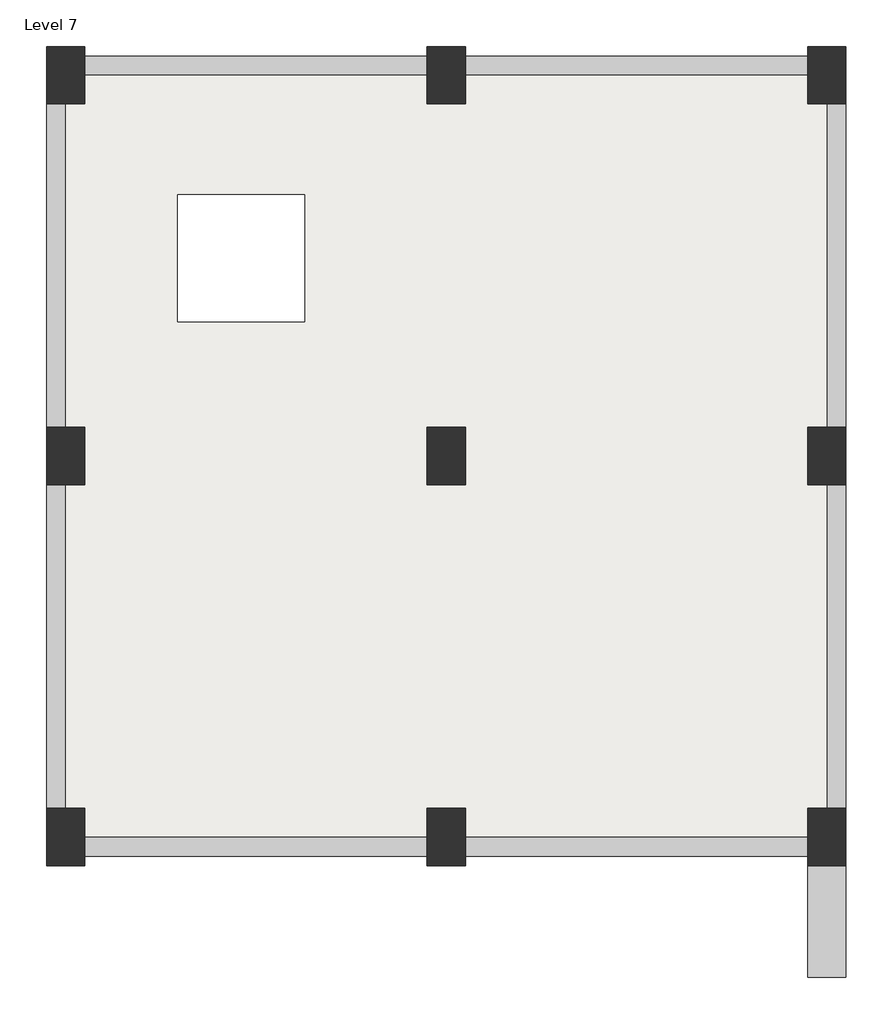
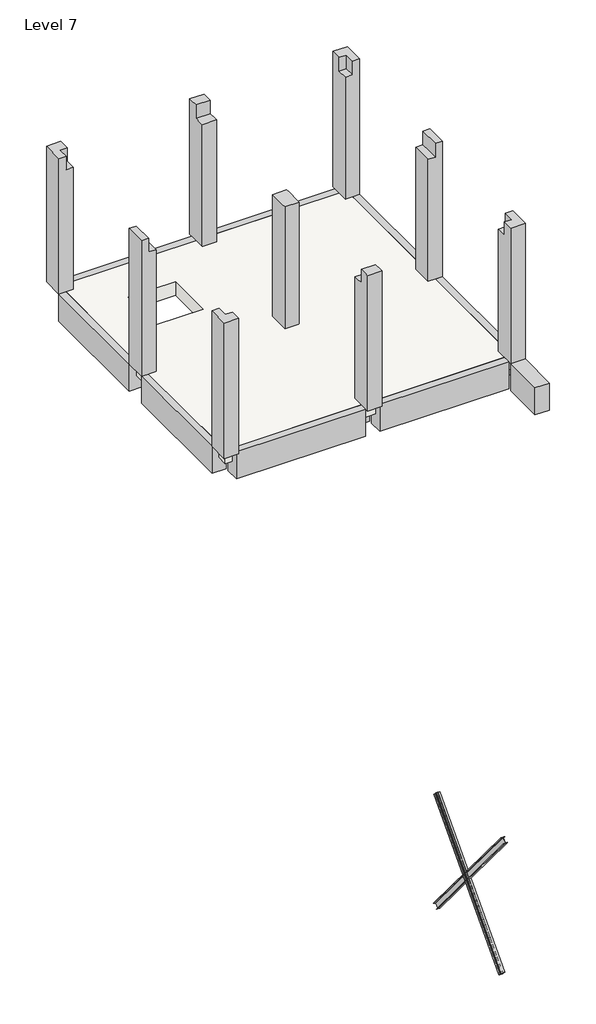
# One storey: 9 columns, 7 beams, 2 members, 1 slab.
"""IFC4 building model written with IfcOpenShell, lengths in millimetres."""

from ifc_helpers import new_model, si_unit, frame, origin, place, context, project, spatial, polyline, outline, extrude, faceted_brep, transform, mapped, element, save
from components import ub_universal_beams_ub127x76x13_5fda7735, ub_universal_beams_ub127x76x13_96cbbb94

model = new_model("IFC4")

# Units and contexts
model_context = context("Model", 3, world=origin())
ifc_project = project(units=[si_unit("LENGTHUNIT", "METRE", prefix="MILLI")], contexts=[model_context])

# Site, building, storey
site = spatial("IfcSite", under=ifc_project)
building = spatial("IfcBuilding", under=site)
storey = spatial("IfcBuildingStorey", under=building, Name="Level 7", Elevation=18000.0)

# Beams
placement = place(None, origin())
element("IfcBeam", 1, ObjectType="Concrete-Rectangular Beam : 300 x 600mm", at=placement, inside=storey, context=model_context, shape_type="SweptSolid", body=[
    extrude(outline(polyline([(526.3372902, 17400.0), (226.3372902, 17400.0), (226.3372902, 17700.0), (376.3372902, 17700.0), (376.3372902, 18000.0), (526.3372902, 18000.0), (526.3372902, 17400.0)])), frame((2068.7595868, 0.0, 0.0), z_axis=(1.0, 0.0, 0.0), x_axis=(0.0, 1.0, 0.0)), (0.0, 0.0, 1.0), 2700.0),
    extrude(outline(polyline([(526.3372902, 17400.0), (226.3372902, 17400.0), (226.3372902, 17700.0), (376.3372902, 17700.0), (376.3372902, 18000.0), (526.3372902, 18000.0), (526.3372902, 17400.0)])), frame((-931.2404132, 0.0, 0.0), z_axis=(1.0, 0.0, 0.0), x_axis=(0.0, 1.0, 0.0)), (0.0, 0.0, 1.0), 2700.0),
])
element("IfcBeam", 2, ObjectType="Concrete-Rectangular Beam : 300 x 600mm", at=placement, inside=storey, context=model_context, shape_type="SweptSolid", body=[
    extrude(outline(polyline([(17400.0, 5068.7595868), (18000.0, 5068.7595868), (18000.0, 4918.7595868), (17700.0, 4918.7595868), (17700.0, 4768.7595868), (17400.0, 4768.7595868), (17400.0, 5068.7595868)])), frame((0.0, -2398.6627098, 0.0), z_axis=(0.0, 1.0, 0.0), x_axis=(0.0, 0.0, 1.0)), (0.0, 0.0, 1.0), 2550.0),
    extrude(outline(polyline([(17400.0, 5068.7595868), (18000.0, 5068.7595868), (18000.0, 4918.7595868), (17700.0, 4918.7595868), (17700.0, 4768.7595868), (17400.0, 4768.7595868), (17400.0, 5068.7595868)])), frame((0.0, -5398.6627098, 0.0), z_axis=(0.0, 1.0, 0.0), x_axis=(0.0, 0.0, 1.0)), (0.0, 0.0, 1.0), 2550.0),
])
element("IfcBeam", 3, ObjectType="Concrete-Rectangular Beam : 300 x 600mm", at=placement, inside=storey, context=model_context, shape_type="SweptSolid", body=[
    extrude(outline(polyline([(-5773.6627098, 17400.0), (-5773.6627098, 18000.0), (-5623.6627098, 18000.0), (-5623.6627098, 17700.0), (-5473.6627098, 17700.0), (-5473.6627098, 17400.0), (-5773.6627098, 17400.0)])), frame((2068.7595868, 0.0, 0.0), z_axis=(1.0, 0.0, 0.0), x_axis=(0.0, 1.0, 0.0)), (0.0, 0.0, 1.0), 2700.0),
    extrude(outline(polyline([(-5773.6627098, 17400.0), (-5773.6627098, 18000.0), (-5623.6627098, 18000.0), (-5623.6627098, 17700.0), (-5473.6627098, 17700.0), (-5473.6627098, 17400.0), (-5773.6627098, 17400.0)])), frame((-931.2404132, 0.0, 0.0), z_axis=(1.0, 0.0, 0.0), x_axis=(0.0, 1.0, 0.0)), (0.0, 0.0, 1.0), 2700.0),
])
element("IfcBeam", 4, ObjectType="Concrete-Rectangular Beam : 300 x 600mm", at=placement, inside=storey, context=model_context, shape_type="SweptSolid", body=[
    extrude(outline(polyline([(18000.0, -1231.2404132), (17400.0, -1231.2404132), (17400.0, -931.2404132), (17700.0, -931.2404132), (17700.0, -1081.2404132), (18000.0, -1081.2404132), (18000.0, -1231.2404132)])), frame((0.0, -5398.6627098, 0.0), z_axis=(0.0, 1.0, 0.0), x_axis=(0.0, 0.0, 1.0)), (0.0, 0.0, 1.0), 2550.0),
    extrude(outline(polyline([(18000.0, -1231.2404132), (17400.0, -1231.2404132), (17400.0, -931.2404132), (17700.0, -931.2404132), (17700.0, -1081.2404132), (18000.0, -1081.2404132), (18000.0, -1231.2404132)])), frame((0.0, -2398.6627098, 0.0), z_axis=(0.0, 1.0, 0.0), x_axis=(0.0, 0.0, 1.0)), (0.0, 0.0, 1.0), 2550.0),
])
element("IfcBeam", 5, ObjectType="Concrete-Rectangular Beam : 300 x 600mm", at=placement, inside=storey, context=model_context, shape_type="SweptSolid", body=[
    extrude(outline(polyline([(2068.7595868, -5398.6627098), (1768.7595868, -5398.6627098), (1768.7595868, -2848.6627098), (2068.7595868, -2848.6627098), (2068.7595868, -5398.6627098)])), frame((0.0, 0.0, 17400.0), z_axis=(0.0, 0.0, 1.0), x_axis=(1.0, 0.0, 0.0)), (0.0, 0.0, 1.0), 300.0),
    extrude(outline(polyline([(1768.7595868, 151.3372902), (2068.7595868, 151.3372902), (2068.7595868, -2398.6627098), (1768.7595868, -2398.6627098), (1768.7595868, 151.3372902)])), frame((0.0, 0.0, 17400.0), z_axis=(0.0, 0.0, 1.0), x_axis=(1.0, 0.0, 0.0)), (0.0, 0.0, 1.0), 300.0),
])
element("IfcBeam", 6, ObjectType="Concrete-Rectangular Beam : 300 x 600mm", at=placement, inside=storey, context=model_context, shape_type="SweptSolid", body=[
    extrude(outline(polyline([(4768.7595868, -2473.6627098), (4768.7595868, -2773.6627098), (2068.7595868, -2773.6627098), (2068.7595868, -2473.6627098), (4768.7595868, -2473.6627098)])), frame((0.0, 0.0, 17400.0), z_axis=(0.0, 0.0, 1.0), x_axis=(1.0, 0.0, 0.0)), (0.0, 0.0, 1.0), 300.0),
    extrude(outline(polyline([(-931.2404132, -2773.6627098), (-931.2404132, -2473.6627098), (1768.7595868, -2473.6627098), (1768.7595868, -2773.6627098), (-931.2404132, -2773.6627098)])), frame((0.0, 0.0, 17400.0), z_axis=(0.0, 0.0, 1.0), x_axis=(1.0, 0.0, 0.0)), (0.0, 0.0, 1.0), 300.0),
])
element("IfcBeam", 7, ObjectType="Concrete-Rectangular Beam : 300 x 600mm", at=placement, inside=storey, context=model_context, shape_type="SweptSolid", body=[
    extrude(outline(polyline([(5068.7595868, -6729.7741204), (4768.7595868, -6729.7741204), (4768.7595868, -5848.6627098), (5068.7595868, -5848.6627098), (5068.7595868, -6729.7741204)])), frame((0.0, 0.0, 17400.0), z_axis=(0.0, 0.0, 1.0), x_axis=(1.0, 0.0, 0.0)), (0.0, 0.0, 1.0), 600.0),
])

# Columns
element("IfcColumn", 8, ObjectType="Concrete-Rectangular-Column : 300 x 450mm", at=placement, inside=storey, context=model_context, shape_type="Brep", body=[
    faceted_brep([(-1231.2404132, -5848.6627098, 21000.0), (-931.2404132, -5848.6627098, 21000.0), (-931.2404132, -5623.6627098, 21000.0), (-1081.2404132, -5623.6627098, 21000.0), (-1081.2404132, -5398.6627098, 21000.0), (-1231.2404132, -5398.6627098, 21000.0), (-1231.2404132, -5848.6627098, 18000.0), (-1231.2404132, -5398.6627098, 18000.0), (-931.2404132, -5398.6627098, 18000.0), (-931.2404132, -5848.6627098, 18000.0), (-931.2404132, -5398.6627098, 20700.0), (-931.2404132, -5623.6627098, 20700.0), (-1081.2404132, -5398.6627098, 20700.0), (-1081.2404132, -5623.6627098, 20700.0)], [[[0, 1, 2, 3, 4, 5]], [[6, 7, 8, 9]], [[1, 0, 6, 9]], [[9, 8, 10, 11, 2, 1]], [[8, 7, 5, 4, 12, 10]], [[0, 5, 7, 6]], [[12, 13, 11, 10]], [[13, 3, 2, 11]], [[3, 13, 12, 4]]]),
])
element("IfcColumn", 9, ObjectType="Concrete-Rectangular-Column : 300 x 450mm", at=placement, inside=storey, context=model_context, shape_type="Brep", body=[
    faceted_brep([(1768.7595868, -5848.6627098, 21000.0), (2068.7595868, -5848.6627098, 21000.0), (2068.7595868, -5773.6627098, 21000.0), (2068.7595868, -5623.6627098, 21000.0), (1768.7595868, -5623.6627098, 21000.0), (1768.7595868, -5773.6627098, 21000.0), (1768.7595868, -5848.6627098, 18000.0), (1768.7595868, -5398.6627098, 18000.0), (2068.7595868, -5398.6627098, 18000.0), (2068.7595868, -5848.6627098, 18000.0), (2068.7595868, -5398.6627098, 20700.0), (2068.7595868, -5473.6627098, 20700.0), (2068.7595868, -5623.6627098, 20700.0), (1768.7595868, -5398.6627098, 20700.0), (1768.7595868, -5623.6627098, 20700.0), (1768.7595868, -5473.6627098, 20700.0)], [[[0, 1, 2, 3, 4, 5]], [[6, 7, 8, 9]], [[1, 0, 6, 9]], [[9, 8, 10, 11, 12, 3, 2, 1]], [[8, 7, 13, 10]], [[7, 6, 0, 5, 4, 14, 15, 13]], [[14, 12, 11, 10, 13, 15]], [[12, 14, 4, 3]]]),
])
element("IfcColumn", 10, ObjectType="Concrete-Rectangular-Column : 300 x 450mm", at=placement, inside=storey, context=model_context, shape_type="Brep", body=[
    faceted_brep([(4768.7595868, -5848.6627098, 21000.0), (5068.7595868, -5848.6627098, 21000.0), (5068.7595868, -5398.6627098, 21000.0), (4918.7595868, -5398.6627098, 21000.0), (4918.7595868, -5623.6627098, 21000.0), (4768.7595868, -5623.6627098, 21000.0), (4768.7595868, -5848.6627098, 18000.0), (4768.7595868, -5398.6627098, 18000.0), (5068.7595868, -5398.6627098, 18000.0), (5068.7595868, -5848.6627098, 18000.0), (4768.7595868, -5398.6627098, 20700.0), (4918.7595868, -5398.6627098, 20700.0), (4768.7595868, -5623.6627098, 20700.0), (4918.7595868, -5623.6627098, 20700.0)], [[[0, 1, 2, 3, 4, 5]], [[6, 7, 8, 9]], [[1, 0, 6, 9]], [[2, 1, 9, 8]], [[8, 7, 10, 11, 3, 2]], [[7, 6, 0, 5, 12, 10]], [[12, 13, 11, 10]], [[13, 4, 3, 11]], [[4, 13, 12, 5]]]),
])
element("IfcColumn", 11, ObjectType="Concrete-Rectangular-Column : 300 x 450mm", at=placement, inside=storey, context=model_context, shape_type="Brep", body=[
    faceted_brep([(-1231.2404132, -2398.6627098, 21000.0), (-1231.2404132, -2848.6627098, 21000.0), (-1081.2404132, -2848.6627098, 21000.0), (-1081.2404132, -2398.6627098, 21000.0), (-1231.2404132, -2848.6627098, 18000.0), (-1231.2404132, -2398.6627098, 18000.0), (-931.2404132, -2398.6627098, 18000.0), (-931.2404132, -2848.6627098, 18000.0), (-931.2404132, -2848.6627098, 20400.0), (-931.2404132, -2848.6627098, 20700.0), (-1081.2404132, -2848.6627098, 20700.0), (-1231.2404132, -2848.6627098, 20400.0), (-931.2404132, -2398.6627098, 20400.0), (-931.2404132, -2398.6627098, 20700.0), (-1231.2404132, -2398.6627098, 20400.0), (-1081.2404132, -2398.6627098, 20700.0)], [[[0, 1, 2, 3]], [[4, 5, 6, 7]], [[4, 7, 8, 9, 10, 2, 1, 11]], [[7, 6, 12, 13, 9, 8]], [[6, 5, 14, 0, 3, 15, 13, 12]], [[1, 0, 14, 5, 4, 11]], [[15, 10, 9, 13]], [[10, 15, 3, 2]]]),
])
element("IfcColumn", 12, ObjectType="Concrete-Rectangular-Column : 300 x 450mm", at=placement, inside=storey, context=model_context, shape_type="Brep", body=[
    faceted_brep([(1768.7595868, -2848.6627098, 18000.0), (1768.7595868, -2398.6627098, 18000.0), (2068.7595868, -2398.6627098, 18000.0), (2068.7595868, -2848.6627098, 18000.0), (2068.7595868, -2848.6627098, 20400.0), (2068.7595868, -2848.6627098, 20700.0), (1768.7595868, -2848.6627098, 20700.0), (1768.7595868, -2848.6627098, 20400.0), (2068.7595868, -2398.6627098, 20400.0), (2068.7595868, -2398.6627098, 20700.0), (2068.7595868, -2473.6627098, 20700.0), (2068.7595868, -2773.6627098, 20700.0), (1768.7595868, -2398.6627098, 20400.0), (1768.7595868, -2398.6627098, 20700.0), (1768.7595868, -2773.6627098, 20700.0), (1768.7595868, -2473.6627098, 20700.0)], [[[0, 1, 2, 3]], [[0, 3, 4, 5, 6, 7]], [[3, 2, 8, 9, 10, 11, 5, 4]], [[2, 1, 12, 13, 9, 8]], [[1, 0, 7, 6, 14, 15, 13, 12]], [[6, 5, 11, 10, 9, 13, 15, 14]]]),
])
element("IfcColumn", 13, ObjectType="Concrete-Rectangular-Column : 300 x 450mm", at=placement, inside=storey, context=model_context, shape_type="Brep", body=[
    faceted_brep([(5068.7595868, -2848.6627098, 21000.0), (5068.7595868, -2398.6627098, 21000.0), (4918.7595868, -2398.6627098, 21000.0), (4918.7595868, -2848.6627098, 21000.0), (4768.7595868, -2848.6627098, 18000.0), (4768.7595868, -2398.6627098, 18000.0), (5068.7595868, -2398.6627098, 18000.0), (5068.7595868, -2848.6627098, 18000.0), (5068.7595868, -2848.6627098, 20400.0), (4918.7595868, -2848.6627098, 20700.0), (4768.7595868, -2848.6627098, 20700.0), (4768.7595868, -2848.6627098, 20400.0), (5068.7595868, -2398.6627098, 20400.0), (4768.7595868, -2398.6627098, 20400.0), (4768.7595868, -2398.6627098, 20700.0), (4918.7595868, -2398.6627098, 20700.0)], [[[0, 1, 2, 3]], [[4, 5, 6, 7]], [[4, 7, 8, 0, 3, 9, 10, 11]], [[1, 0, 8, 7, 6, 12]], [[6, 5, 13, 14, 15, 2, 1, 12]], [[5, 4, 11, 10, 14, 13]], [[9, 15, 14, 10]], [[15, 9, 3, 2]]]),
])
element("IfcColumn", 14, ObjectType="Concrete-Rectangular-Column : 300 x 450mm", at=placement, inside=storey, context=model_context, shape_type="Brep", body=[
    faceted_brep([(-931.2404132, 601.3372902, 21000.0), (-1231.2404132, 601.3372902, 21000.0), (-1231.2404132, 151.3372902, 21000.0), (-1081.2404132, 151.3372902, 21000.0), (-1081.2404132, 376.3372902, 21000.0), (-931.2404132, 376.3372902, 21000.0), (-1231.2404132, 151.3372902, 18000.0), (-1231.2404132, 601.3372902, 18000.0), (-931.2404132, 601.3372902, 18000.0), (-931.2404132, 151.3372902, 18000.0), (-931.2404132, 151.3372902, 20700.0), (-1081.2404132, 151.3372902, 20700.0), (-931.2404132, 376.3372902, 20700.0), (-1081.2404132, 376.3372902, 20700.0)], [[[0, 1, 2, 3, 4, 5]], [[6, 7, 8, 9]], [[6, 9, 10, 11, 3, 2]], [[9, 8, 0, 5, 12, 10]], [[1, 0, 8, 7]], [[2, 1, 7, 6]], [[12, 13, 11, 10]], [[13, 4, 3, 11]], [[4, 13, 12, 5]]]),
])
element("IfcColumn", 15, ObjectType="Concrete-Rectangular-Column : 300 x 450mm", at=placement, inside=storey, context=model_context, shape_type="Brep", body=[
    faceted_brep([(2068.7595868, 601.3372902, 21000.0), (1768.7595868, 601.3372902, 21000.0), (1768.7595868, 526.3372902, 21000.0), (1768.7595868, 376.3372902, 21000.0), (2068.7595868, 376.3372902, 21000.0), (2068.7595868, 526.3372902, 21000.0), (1768.7595868, 151.3372902, 18000.0), (1768.7595868, 601.3372902, 18000.0), (2068.7595868, 601.3372902, 18000.0), (2068.7595868, 151.3372902, 18000.0), (2068.7595868, 151.3372902, 20700.0), (1768.7595868, 151.3372902, 20700.0), (2068.7595868, 376.3372902, 20700.0), (2068.7595868, 226.3372902, 20700.0), (1768.7595868, 226.3372902, 20700.0), (1768.7595868, 376.3372902, 20700.0)], [[[0, 1, 2, 3, 4, 5]], [[6, 7, 8, 9]], [[6, 9, 10, 11]], [[9, 8, 0, 5, 4, 12, 13, 10]], [[1, 0, 8, 7]], [[7, 6, 11, 14, 15, 3, 2, 1]], [[12, 15, 14, 11, 10, 13]], [[15, 12, 4, 3]]]),
])
element("IfcColumn", 16, ObjectType="Concrete-Rectangular-Column : 300 x 450mm", at=placement, inside=storey, context=model_context, shape_type="Brep", body=[
    faceted_brep([(5068.7595868, 151.3372902, 21000.0), (5068.7595868, 601.3372902, 21000.0), (4768.7595868, 601.3372902, 21000.0), (4768.7595868, 376.3372902, 21000.0), (4918.7595868, 376.3372902, 21000.0), (4918.7595868, 151.3372902, 21000.0), (4768.7595868, 151.3372902, 18000.0), (4768.7595868, 601.3372902, 18000.0), (5068.7595868, 601.3372902, 18000.0), (5068.7595868, 151.3372902, 18000.0), (4918.7595868, 151.3372902, 20700.0), (4768.7595868, 151.3372902, 20700.0), (4768.7595868, 376.3372902, 20700.0), (4918.7595868, 376.3372902, 20700.0)], [[[0, 1, 2, 3, 4, 5]], [[6, 7, 8, 9]], [[6, 9, 0, 5, 10, 11]], [[1, 0, 9, 8]], [[2, 1, 8, 7]], [[7, 6, 11, 12, 3, 2]], [[13, 12, 11, 10]], [[4, 13, 10, 5]], [[13, 4, 3, 12]]]),
])

# Members
ub_universal_beams_ub127x76x13_shape = ub_universal_beams_ub127x76x13_5fda7735(model_context)
element("IfcMember", 17, ObjectType="UB-Universal Beams : UB127x76x13", at=placement, inside=storey, context=model_context, shape_type="MappedRepresentation", body=[
    mapped(ub_universal_beams_ub127x76x13_shape, transform((4918.7595868, -3987.3365723, 5466.3104182), x_axis=(0.0, 0.6408125760238288, -0.7676973638157842), y_axis=(-1.0, 0.0, 0.0), z_axis=(0.0, 0.7676973638157842, 0.6408125760238288))),
])
ub_universal_beams_ub127x76x13_2_shape = ub_universal_beams_ub127x76x13_96cbbb94(model_context)
element("IfcMember", 18, ObjectType="UB-Universal Beams : UB127x76x13", at=placement, inside=storey, context=model_context, shape_type="MappedRepresentation", body=[
    mapped(ub_universal_beams_ub127x76x13_2_shape, transform((4918.7595868, -3946.516498, 5534.1249429), x_axis=(0.0, -0.6780160909774431, -0.7350470599734874), y_axis=(1.0, 0.0, 0.0), z_axis=(0.0, -0.7350470599734874, 0.6780160909774431))),
])

# Slab
element("IfcSlab", 19, ObjectType="Generic 300mm", at=placement, inside=storey, context=model_context, shape_type="Brep", body=[
    faceted_brep([(4918.7595868, 376.3372902, 17700.0), (4918.7595868, 151.3372902, 17700.0), (4918.7595868, -2398.6627098, 17700.0), (4918.7595868, -2848.6627098, 17700.0), (4918.7595868, -5398.6627098, 17700.0), (4918.7595868, -5623.6627098, 17700.0), (4768.7595868, -5623.6627098, 17700.0), (2068.7595868, -5623.6627098, 17700.0), (1768.7595868, -5623.6627098, 17700.0), (-931.2404132, -5623.6627098, 17700.0), (-1081.2404132, -5623.6627098, 17700.0), (-1081.2404132, -5398.6627098, 17700.0), (-1081.2404132, -2848.6627098, 17700.0), (-1081.2404132, -2398.6627098, 17700.0), (-1081.2404132, 151.3372902, 17700.0), (-1081.2404132, 376.3372902, 17700.0), (-931.2404132, 376.3372902, 17700.0), (1768.7595868, 376.3372902, 17700.0), (2068.7595868, 376.3372902, 17700.0), (4768.7595868, 376.3372902, 17700.0), (-198.5229478, -1566.5574371, 17700.0), (801.4770522, -1566.5574371, 17700.0), (801.4770522, -566.5574371, 17700.0), (-198.5229478, -566.5574371, 17700.0), (4918.7595868, -5623.6627098, 18000.0), (4918.7595868, -5398.6627098, 18000.0), (4918.7595868, -2848.6627098, 18000.0), (4918.7595868, -2398.6627098, 18000.0), (4918.7595868, 151.3372902, 18000.0), (4918.7595868, 376.3372902, 18000.0), (4768.7595868, 376.3372902, 18000.0), (2068.7595868, 376.3372902, 18000.0), (1768.7595868, 376.3372902, 18000.0), (-931.2404132, 376.3372902, 18000.0), (-1081.2404132, 376.3372902, 18000.0), (-1081.2404132, 151.3372902, 18000.0), (-1081.2404132, -2398.6627098, 18000.0), (-1081.2404132, -2848.6627098, 18000.0), (-1081.2404132, -5398.6627098, 18000.0), (-1081.2404132, -5623.6627098, 18000.0), (-931.2404132, -5623.6627098, 18000.0), (1768.7595868, -5623.6627098, 18000.0), (2068.7595868, -5623.6627098, 18000.0), (4768.7595868, -5623.6627098, 18000.0), (801.4770522, -1566.5574371, 18000.0), (-198.5229478, -1566.5574371, 18000.0), (-198.5229478, -566.5574371, 18000.0), (801.4770522, -566.5574371, 18000.0)], [[[0, 1, 2, 3, 4, 5, 6, 7, 8, 9, 10, 11, 12, 13, 14, 15, 16, 17, 18, 19], [20, 21, 22, 23]], [[24, 25, 26, 27, 28, 29, 30, 31, 32, 33, 34, 35, 36, 37, 38, 39, 40, 41, 42, 43], [44, 45, 46, 47]], [[5, 4, 3, 2, 1, 0, 29, 28, 27, 26, 25, 24]], [[10, 9, 8, 7, 6, 5, 24, 43, 42, 41, 40, 39]], [[15, 14, 13, 12, 11, 10, 39, 38, 37, 36, 35, 34]], [[0, 19, 18, 17, 16, 15, 34, 33, 32, 31, 30, 29]], [[20, 45, 44, 21]], [[21, 44, 47, 22]], [[22, 47, 46, 23]], [[45, 20, 23, 46]]]),
])

save(model, "model.ifc")

# Revit data of these elements
# Type "Concrete-Rectangular Beam : 300 x 600mm"
#   Length [instance default] = 1.524 m
#   b = 0.3 m
#   h = 0.6 m
#   Structural Material [instance default] = Concrete, Cast-in-Place gray
#   Assembly Code = ""
# Type "Concrete-Rectangular-Column : 300 x 450mm"
#   b = 0.3 m
#   h = 0.45 m
#   Structural Material [instance default] = Concrete, Cast-in-Place gray
# Type "UB-Universal Beams : UB127x76x13"
#   Section Name Key = "UB127X76X13"
#   Width = 7.6 cm
#   Web Thickness = 0.4 cm
#   Web Fillet = 0.76 cm
#   Warping Constant = 2000.0 cm⁶
#   Torsional Moment of Inertia = 2.85 cm⁴
#   Section Area = 16.5 cm²
#   Plastic Modulus weak axis = 22.6 cm³
#   Plastic Modulus strong axis = 84.2 cm³
#   Nominal Weight = 13.00 kgf/m
#   Moment of Inertia weak axis = 55.70 cm⁴
#   Moment of Inertia strong axis = 473.00 cm⁴
#   Height = 12.7 cm
#   Flange Thickness = 0.76 cm
#   Elastic Modulus weak axis = 14.7 cm³
#   Elastic Modulus strong axis = 74.6 cm³
#   Centroid Vertical = 6.35 cm
#   Centroid Horizontal = 3.8 cm
#   Bolt Spacing = 4.0 cm
#   Length [instance default] = 1.5 m
#   Structural Material [instance default] = Metal - Steel 43-275
#   Type Comments = ""
#   Assembly Code = ""
# Type "Generic 300mm"
#   Function = 0
#   Layers, outside or top first: 0.3 m no material (function 1)
# Elements 1, 2, 3, 4, 5, 6, 7 (IfcBeam, "Concrete-Rectangular Beam : 300 x 600mm")
#   Structural Material = Concrete, Cast-in-Place gray
#   Phase Created = New Construction
#   Materials on its faces: "Concrete, Cast-in-Place gray"
# Elements 8, 9, 10, 11, 12, 13, 14, 15, 16 (IfcColumn, "Concrete-Rectangular-Column : 300 x 450mm")
#   Structural Material = Concrete, Cast-in-Place gray
#   Phase Created = New Construction
#   Materials on its faces: "Concrete, Cast-in-Place gray"
# Elements 17, 18 (IfcMember, "UB-Universal Beams : UB127x76x13")
#   Structural Material = Metal - Steel 43-275
#   Phase Created = New Construction
#   Materials on its faces: "Metal - Steel 43-275"
# Element 19 (IfcSlab, "Generic 300mm")
#   Height Offset From Level = 0 m
#   built-in parameter 1001954 = 1
#   Phase Created = New Construction
#   Materials on its faces: "Default Floor"
# Materials
#   "Concrete, Cast-in-Place gray": class "Concrete", colour RGB 192 192 192, transparency 0, Description = "Cast-in-place concrete", Cost = 0
#   "Metal - Steel 43-275": class "Metal", colour RGB 247 247 247, transparency 0, Cost = 0
#   "Default Floor": colour RGB 127 127 127, transparency 0, Cost = 0
